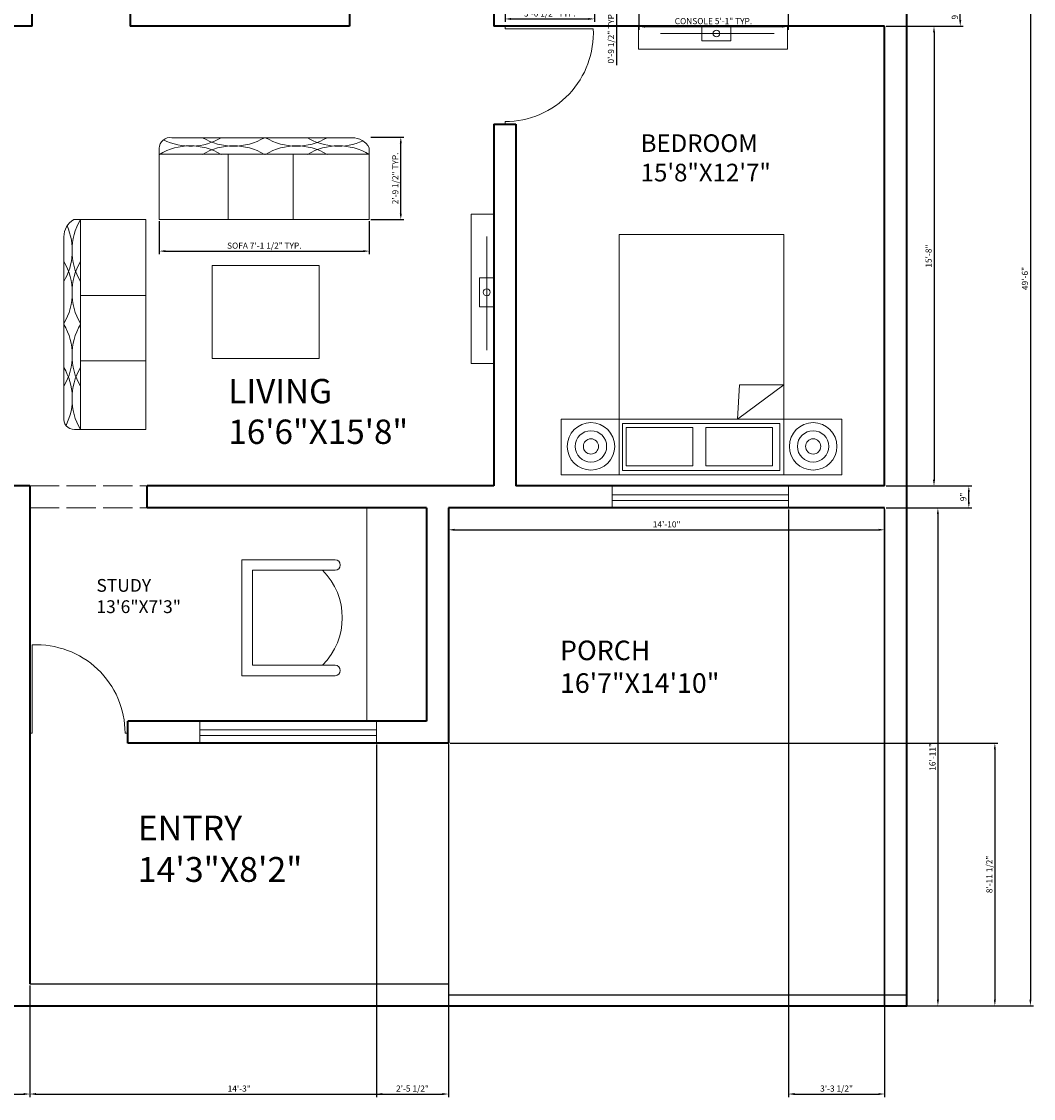
# Model space of a CAD drawing. Units: inches. Extents: x 808 to 1433, y 803 to 1556.
# Tile 2 of 4: x 1020 to 1433, y 803 to 1243. Entities that reach past the tile are written whole.
import ezdxf

# ---------------------------------------------------------------- set-up
doc = ezdxf.new("R2010")
doc.units = ezdxf.units.IN
doc.linetypes.add('ACAD_ISO02W100', pattern=[15, 12, -3])
for name, color, linetype, lineweight in [('A-ANNO-DIMS', 7, 'Continuous', 13), ('A-AREA-IDEN', 7, 'Continuous', 18), ('A-FLOR', 7, 'Continuous', 25), ('A-FLOR-CASE', 7, 'Continuous', 18), ('A-FLOR-OVHD', 7, 'ACAD_ISO02W100', 13), ('A-WALL', 7, 'Continuous', 35)]:
    doc.layers.add(name, color=color, linetype=linetype, lineweight=lineweight)
for name, color, linetype, lineweight, true_color in [('A-DOOR', 251, 'Continuous', 18, 0x636466), ('A-FURN', 251, 'Continuous', 13, 0x636466), ('A-GLAZ', 251, 'Continuous', 18, 0x636466)]:
    doc.layers.add(name, color=color, linetype=linetype, lineweight=lineweight, true_color=true_color)
doc.styles.get("Standard").update_dxf_attribs({"font": 'arial.ttf'})
doc.dimstyles.new('ISO-25', dxfattribs={"dimtxt": 2.5, "dimasz": 2.5, "dimexe": 1.25, "dimexo": 0.625, "dimtad": 1, "dimdec": 0, "dimlunit": 3, "dimtxsty": 'Standard', "dimcen": 2.5, "dimadec": 0, "dimazin": 0, "dimtfac": 1, "dimtdec": 0, "dimtmove": 0, "dimatfit": 3, "dimfxl": 1, "dimarcsym": 0})

# ---------------------------------------------------------------- blocks, each defined once
blk = doc.blocks.new('*D2')
at = {"layer": 'A-ANNO-DIMS', "color": 0, "lineweight": -2, "transparency": 16777216}
for p, q in [((1381.5, 1435.07), (1432.64, 1435.07)), ((1431.39, 1432.57), (1431.39, 843.57)), ((1381.5, 841.07), (1432.64, 841.07))]:
    blk.add_line(p, q, dxfattribs=at)
at = {"layer": 'A-ANNO-DIMS', "color": 0, "transparency": 16777216}
for points in [[(1430.97, 1432.57), (1431.8, 1432.57), (1431.39, 1435.07)], [(1430.97, 843.57), (1431.8, 843.57), (1431.39, 841.07)]]:
    blk.add_solid(points, dxfattribs=at)
at = {"layer": 'Defpoints', "color": 0, "transparency": 16777216}
for p in [(1380.88, 1435.07), (1380.88, 841.07), (1431.39, 841.07)]:
    blk.add_point(p, dxfattribs=at)
at = {"layer": 'A-ANNO-DIMS', "color": 0, "transparency": 16777216, "insert": (1429.48, 1138.07), "char_height": 2.5, "attachment_point": 5, "rotation": 90}
blk.add_mtext('49\'-6"', dxfattribs=at)
blk = doc.blocks.new('*D21')
at = {"layer": 'A-ANNO-DIMS', "color": 0, "lineweight": -2, "transparency": 16777216}
for p, q in [((1372.5, 1250.07), (1404, 1250.07)), ((1402.75, 1243.57), (1402.75, 1247.57)), ((1372.5, 1241.07), (1404, 1241.07))]:
    blk.add_line(p, q, dxfattribs=at)
at = {"layer": 'A-ANNO-DIMS', "color": 0, "transparency": 16777216}
for points in [[(1402.33, 1247.57), (1403.16, 1247.57), (1402.75, 1250.07)], [(1402.33, 1243.57), (1403.16, 1243.57), (1402.75, 1241.07)]]:
    blk.add_solid(points, dxfattribs=at)
at = {"layer": 'Defpoints', "color": 0, "transparency": 16777216}
for p in [(1371.88, 1250.07), (1402.75, 1250.07), (1371.88, 1241.07)]:
    blk.add_point(p, dxfattribs=at)
at = {"layer": 'A-ANNO-DIMS', "color": 0, "transparency": 16777216, "insert": (1400.85, 1245.57), "char_height": 2.5, "attachment_point": 5, "rotation": 90}
blk.add_mtext('9"', dxfattribs=at)
blk = doc.blocks.new('*D22')
at = {"layer": 'A-ANNO-DIMS', "color": 0, "lineweight": -2, "transparency": 16777216}
for p, q in [((1372.5, 1053.37), (1407.5, 1053.37)), ((1406.25, 1046.87), (1406.25, 1050.87)), ((1372.5, 1044.37), (1407.5, 1044.37))]:
    blk.add_line(p, q, dxfattribs=at)
at = {"layer": 'A-ANNO-DIMS', "color": 0, "transparency": 16777216}
for points in [[(1405.83, 1050.87), (1406.66, 1050.87), (1406.25, 1053.37)], [(1405.83, 1046.87), (1406.66, 1046.87), (1406.25, 1044.37)]]:
    blk.add_solid(points, dxfattribs=at)
at = {"layer": 'Defpoints', "color": 0, "transparency": 16777216}
for p in [(1371.88, 1053.37), (1406.25, 1053.37), (1371.88, 1044.37)]:
    blk.add_point(p, dxfattribs=at)
at = {"layer": 'A-ANNO-DIMS', "color": 0, "transparency": 16777216, "insert": (1404.34, 1048.87), "char_height": 2.5, "attachment_point": 5, "rotation": 90}
blk.add_mtext('9"', dxfattribs=at)
blk = doc.blocks.new('*D23')
at = {"layer": 'A-ANNO-DIMS', "color": 0, "lineweight": -2, "transparency": 16777216}
for p, q in [((1193.88, 1043.75), (1193.88, 1034.21)), ((1371.88, 1043.75), (1371.88, 1034.21)), ((1196.38, 1035.46), (1369.38, 1035.46))]:
    blk.add_line(p, q, dxfattribs=at)
at = {"layer": 'A-ANNO-DIMS', "color": 0, "transparency": 16777216}
for points in [[(1196.38, 1035.88), (1196.38, 1035.04), (1193.88, 1035.46)], [(1369.38, 1035.88), (1369.38, 1035.04), (1371.88, 1035.46)]]:
    blk.add_solid(points, dxfattribs=at)
at = {"layer": 'Defpoints', "color": 0, "transparency": 16777216}
for p in [(1193.88, 1044.37), (1371.88, 1044.37), (1371.88, 1035.46)]:
    blk.add_point(p, dxfattribs=at)
at = {"layer": 'A-ANNO-DIMS', "color": 0, "transparency": 16777216, "insert": (1282.88, 1037.36), "char_height": 2.5, "attachment_point": 5}
blk.add_mtext('14\'-10"', dxfattribs=at)
blk = doc.blocks.new('*D24')
at = {"layer": 'A-ANNO-DIMS', "color": 0, "lineweight": -2, "transparency": 16777216}
for p, q in [((1381.5, 1044.37), (1394.88, 1044.37)), ((1393.63, 1041.87), (1393.63, 843.57)), ((1381.5, 841.07), (1394.88, 841.07))]:
    blk.add_line(p, q, dxfattribs=at)
at = {"layer": 'A-ANNO-DIMS', "color": 0, "transparency": 16777216}
for points in [[(1393.21, 1041.87), (1394.04, 1041.87), (1393.63, 1044.37)], [(1393.21, 843.57), (1394.04, 843.57), (1393.63, 841.07)]]:
    blk.add_solid(points, dxfattribs=at)
at = {"layer": 'Defpoints', "color": 0, "transparency": 16777216}
for p in [(1380.88, 1044.37), (1380.88, 841.07), (1393.63, 841.07)]:
    blk.add_point(p, dxfattribs=at)
at = {"layer": 'A-ANNO-DIMS', "color": 0, "transparency": 16777216, "insert": (1391.73, 942.72), "char_height": 2.5, "attachment_point": 5, "rotation": 90}
blk.add_mtext('16\'-11"', dxfattribs=at)
blk = doc.blocks.new('*D25')
at = {"layer": 'A-ANNO-DIMS', "color": 0, "lineweight": -2, "transparency": 16777216}
for p, q in [((1381.5, 1241.07), (1393.29, 1241.07)), ((1392.04, 1238.57), (1392.04, 1055.87)), ((1381.5, 1053.37), (1393.29, 1053.37))]:
    blk.add_line(p, q, dxfattribs=at)
at = {"layer": 'A-ANNO-DIMS', "color": 0, "transparency": 16777216}
for points in [[(1391.62, 1238.57), (1392.45, 1238.57), (1392.04, 1241.07)], [(1391.62, 1055.87), (1392.45, 1055.87), (1392.04, 1053.37)]]:
    blk.add_solid(points, dxfattribs=at)
at = {"layer": 'Defpoints', "color": 0, "transparency": 16777216}
for p in [(1380.88, 1241.07), (1380.88, 1053.37), (1392.04, 1053.37)]:
    blk.add_point(p, dxfattribs=at)
at = {"layer": 'A-ANNO-DIMS', "color": 0, "transparency": 16777216, "insert": (1390.14, 1147.22), "char_height": 2.5, "attachment_point": 5, "rotation": 90}
blk.add_mtext('15\'-8"', dxfattribs=at)
blk = doc.blocks.new('BED-DOUBLE-NIGHTSTANDS')
for p, q in [((23.66, 75.46), (90.98, 75.46)), ((72.01, 75.46), (90.98, 61.39)), ((72.82, 61.39), (72.01, 75.46)), ((90.98, 61.39), (72.82, 61.39))]:
    blk.add_line(p, q)
for points in [[(23.66, 98.16), (0, 98.16), (0, 75.46), (23.66, 75.46)], [(23.66, 0), (90.98, 0), (90.98, 98.16), (23.66, 98.16)], [(114.63, 98.16), (90.98, 98.16), (90.98, 75.46), (114.63, 75.46)], [(25.04, 77.24), (89.23, 77.24), (89.23, 96.41), (25.04, 96.41)], [(26.57, 78.89), (53.84, 78.89), (53.84, 94.57), (26.57, 94.57)], [(59.07, 78.89), (86.35, 78.89), (86.35, 94.57), (59.07, 94.57)]]:
    blk.add_lwpolyline(points, close=True)
for centre, radius in [((12.19, 86.58), 9.7), ((12.19, 86.58), 6.41), ((102.89, 86.58), 9.7), ((102.89, 86.58), 6.41), ((12.19, 86.58), 3.11), ((102.89, 86.58), 3.11)]:
    blk.add_circle(centre, radius)
blk = doc.blocks.new('SOFA-3SEAT')
for p, q in [((78.71, 33.47), (5.06, 33.47)), ((0, 29.12), (0, 26.67)), ((28.12, 0), (28.12, 26.67)), ((54.7, 0), (54.7, 26.67)), ((85.72, 26.67), (85.72, 29.39))]:
    blk.add_line(p, q)
blk.add_lwpolyline([(0, 0), (85.72, 0), (85.72, 26.67), (0, 26.67)], close=True)
for centre, radius, start, end in [((4.4, 29.12), 4.4, 81.2898, 180), ((12.64, 54.74), 24.74, 243.6614, 300.7197), ((30.31, 54.74), 24.74, 239.2803, 300.7197), ((55.93, 54.74), 24.74, 239.2803, 300.7197), ((73.08, 54.74), 24.74, 239.2803, 294.0125), ((78.71, 25.4), 8.06, 29.6577, 90), ((12.64, 5.39), 24.74, 59.2803, 120.7197), ((30.31, 5.39), 24.74, 59.2803, 120.7197), ((55.93, 5.39), 24.74, 59.2803, 120.7197), ((73.08, 5.39), 24.74, 59.2803, 120.7197)]:
    blk.add_arc(centre, radius, start, end)
blk = doc.blocks.new('MEDIA-CONSOLE')
for q in [(6.39, 51.9), (6.39, 5.5)]:
    blk.add_line((6.39, 23.14), q)
for points in [[(9.33, 60.92), (0, 60.92), (0, 0), (9.33, 0)], [(9.33, 35.01), (3.45, 35.01), (3.45, 23.14), (9.33, 23.14)]]:
    blk.add_lwpolyline(points, close=True)
blk.add_circle((6.39, 29.07), 1.39)
blk = doc.blocks.new('WIN-72')
for points in [[(0, 0), (72, 0), (72, 9), (0, 9)], [(0, 5.39), (72, 5.39), (72, 3.12), (0, 3.12)]]:
    blk.add_lwpolyline(points, close=True)
blk = doc.blocks.new('DOOR-40')
for p, q in [((0, 40), (0, 38.9)), ((0, 1), (36, 1)), ((0, 1), (0, 0))]:
    blk.add_line(p, q)
blk.add_arc((0, 2.85), 36.05, 357.0527, 90)
blk = doc.blocks.new('*D48')
at = {"layer": 'A-ANNO-DIMS', "color": 0, "lineweight": -2, "transparency": 16777216}
for p, q in [((1216.91, 1249.44), (1216.91, 1242.82)), ((1253.42, 1249.44), (1253.42, 1242.82)), ((1219.41, 1244.07), (1250.92, 1244.07))]:
    blk.add_line(p, q, dxfattribs=at)
at = {"layer": 'A-ANNO-DIMS', "color": 0, "transparency": 16777216}
for points in [[(1219.41, 1244.48), (1219.41, 1243.65), (1216.91, 1244.07)], [(1250.92, 1244.48), (1250.92, 1243.65), (1253.42, 1244.07)]]:
    blk.add_solid(points, dxfattribs=at)
at = {"layer": 'Defpoints', "color": 0, "transparency": 16777216}
for p in [(1216.91, 1250.07), (1253.42, 1250.07), (1253.42, 1244.07)]:
    blk.add_point(p, dxfattribs=at)
at = {"layer": 'A-ANNO-DIMS', "color": 0, "transparency": 16777216, "insert": (1235.17, 1245.98), "char_height": 2.5, "attachment_point": 5}
blk.add_mtext('3\'-0 1/2" TYP.', dxfattribs=at)
blk = doc.blocks.new('*D55')
at = {"layer": 'A-ANNO-DIMS', "color": 0, "lineweight": -2, "transparency": 16777216}
for p, q in [((1075.78, 1161.49), (1075.78, 1148.01)), ((1161.5, 1161.49), (1161.5, 1148.01)), ((1078.28, 1149.26), (1159, 1149.26))]:
    blk.add_line(p, q, dxfattribs=at)
at = {"layer": 'A-ANNO-DIMS', "color": 0, "transparency": 16777216}
for points in [[(1078.28, 1149.67), (1078.28, 1148.84), (1075.78, 1149.26)], [(1159, 1149.67), (1159, 1148.84), (1161.5, 1149.26)]]:
    blk.add_solid(points, dxfattribs=at)
at = {"layer": 'Defpoints', "color": 0, "transparency": 16777216}
for p in [(1075.78, 1162.11), (1161.5, 1162.11), (1161.5, 1149.26)]:
    blk.add_point(p, dxfattribs=at)
at = {"layer": 'A-ANNO-DIMS', "color": 0, "transparency": 16777216, "insert": (1118.64, 1151.17), "char_height": 2.5, "attachment_point": 5}
blk.add_mtext('SOFA 7\'-1 1/2" TYP.', dxfattribs=at)
blk = doc.blocks.new('*D56')
at = {"layer": 'A-ANNO-DIMS', "color": 0, "lineweight": -2, "transparency": 16777216}
for p, q in [((1162.13, 1195.78), (1175.61, 1195.78)), ((1174.36, 1164.61), (1174.36, 1193.28)), ((1162.13, 1162.11), (1175.61, 1162.11))]:
    blk.add_line(p, q, dxfattribs=at)
at = {"layer": 'A-ANNO-DIMS', "color": 0, "transparency": 16777216}
for points in [[(1173.94, 1193.28), (1174.78, 1193.28), (1174.36, 1195.78)], [(1173.94, 1164.61), (1174.78, 1164.61), (1174.36, 1162.11)]]:
    blk.add_solid(points, dxfattribs=at)
at = {"layer": 'Defpoints', "color": 0, "transparency": 16777216}
for p in [(1161.5, 1195.78), (1174.36, 1195.78), (1161.5, 1162.11)]:
    blk.add_point(p, dxfattribs=at)
at = {"layer": 'A-ANNO-DIMS', "color": 0, "transparency": 16777216, "insert": (1172.44, 1178.95), "char_height": 2.5, "attachment_point": 5, "rotation": 90}
blk.add_mtext('2\'-9 1/2" TYP.', dxfattribs=at)
blk = doc.blocks.new('*D57')
at = {"layer": 'A-ANNO-DIMS', "color": 0, "lineweight": -2, "transparency": 16777216}
for p, q in [((1271.53, 1249.44), (1271.53, 1239.68)), ((1332.45, 1249.44), (1332.45, 1239.68)), ((1274.03, 1240.93), (1329.95, 1240.93))]:
    blk.add_line(p, q, dxfattribs=at)
at = {"layer": 'A-ANNO-DIMS', "color": 0, "transparency": 16777216}
for points in [[(1274.03, 1241.35), (1274.03, 1240.51), (1271.53, 1240.93)], [(1329.95, 1241.35), (1329.95, 1240.51), (1332.45, 1240.93)]]:
    blk.add_solid(points, dxfattribs=at)
at = {"layer": 'Defpoints', "color": 0, "transparency": 16777216}
for p in [(1271.53, 1250.07), (1332.45, 1250.07), (1332.45, 1240.93)]:
    blk.add_point(p, dxfattribs=at)
at = {"layer": 'A-ANNO-DIMS', "color": 0, "transparency": 16777216, "insert": (1301.99, 1242.85), "char_height": 2.5, "attachment_point": 5}
blk.add_mtext('CONSOLE 5\'-1" TYP.', dxfattribs=at)
blk = doc.blocks.new('*D58')
at = {"layer": 'A-ANNO-DIMS', "color": 0, "lineweight": -2, "transparency": 16777216}
for p, q in [((1270.91, 1259.4), (1261.14, 1259.4)), ((1262.39, 1256.9), (1262.39, 1252.57)), ((1270.91, 1250.07), (1261.14, 1250.07)), ((1262.39, 1250.07), (1262.39, 1225.25))]:
    blk.add_line(p, q, dxfattribs=at)
at = {"layer": 'A-ANNO-DIMS', "color": 0, "transparency": 16777216}
for points in [[(1261.98, 1256.9), (1262.81, 1256.9), (1262.39, 1259.4)], [(1261.98, 1252.57), (1262.81, 1252.57), (1262.39, 1250.07)]]:
    blk.add_solid(points, dxfattribs=at)
at = {"layer": 'Defpoints', "color": 0, "transparency": 16777216}
for p in [(1271.53, 1259.4), (1262.39, 1250.07), (1271.53, 1250.07)]:
    blk.add_point(p, dxfattribs=at)
at = {"layer": 'A-ANNO-DIMS', "color": 0, "transparency": 16777216, "insert": (1260.48, 1236.41), "char_height": 2.5, "attachment_point": 5, "rotation": 90}
blk.add_mtext('0\'-9 1/2" TYP.', dxfattribs=at)
blk = doc.blocks.new('*D66')
at = {"layer": 'A-ANNO-DIMS', "color": 0, "lineweight": -2, "transparency": 16777216}
for p, q in [((1022.88, 849.44), (1022.88, 803.82)), ((971.87, 840.44), (971.87, 803.82)), ((974.37, 805.07), (1020.38, 805.07))]:
    blk.add_line(p, q, dxfattribs=at)
at = {"layer": 'A-ANNO-DIMS', "color": 0, "transparency": 16777216}
for points in [[(974.37, 805.48), (974.37, 804.65), (971.87, 805.07)], [(1020.38, 805.48), (1020.38, 804.65), (1022.88, 805.07)]]:
    blk.add_solid(points, dxfattribs=at)
at = {"layer": 'Defpoints', "color": 0, "transparency": 16777216}
for p in [(1022.88, 850.07), (971.87, 841.07), (1022.88, 805.07)]:
    blk.add_point(p, dxfattribs=at)
at = {"layer": 'A-ANNO-DIMS', "color": 0, "transparency": 16777216, "insert": (997.38, 806.97), "char_height": 2.5, "attachment_point": 5}
blk.add_mtext('4\'-3"', dxfattribs=at)
blk = doc.blocks.new('*D67')
at = {"layer": 'A-ANNO-DIMS', "color": 0, "lineweight": -2, "transparency": 16777216}
for p, q in [((1022.88, 849.44), (1022.88, 803.82)), ((1193.88, 840.44), (1193.88, 803.82)), ((1025.38, 805.07), (1191.38, 805.07))]:
    blk.add_line(p, q, dxfattribs=at)
at = {"layer": 'A-ANNO-DIMS', "color": 0, "transparency": 16777216}
for points in [[(1025.38, 805.48), (1025.38, 804.65), (1022.88, 805.07)], [(1191.38, 805.48), (1191.38, 804.65), (1193.88, 805.07)]]:
    blk.add_solid(points, dxfattribs=at)
at = {"layer": 'Defpoints', "color": 0, "transparency": 16777216}
for p in [(1022.88, 850.07), (1193.88, 841.07), (1193.88, 805.07)]:
    blk.add_point(p, dxfattribs=at)
at = {"layer": 'A-ANNO-DIMS', "color": 0, "transparency": 16777216, "insert": (1108.38, 806.97), "char_height": 2.5, "attachment_point": 5}
blk.add_mtext('14\'-3"', dxfattribs=at)
blk = doc.blocks.new('*D70')
at = {"layer": 'A-ANNO-DIMS', "color": 0, "lineweight": -2, "transparency": 16777216}
for p, q in [((1164.38, 947.75), (1164.38, 803.82)), ((1193.88, 947.75), (1193.88, 803.82)), ((1166.88, 805.07), (1191.38, 805.07))]:
    blk.add_line(p, q, dxfattribs=at)
at = {"layer": 'A-ANNO-DIMS', "color": 0, "transparency": 16777216}
for points in [[(1166.88, 805.48), (1166.88, 804.65), (1164.38, 805.07)], [(1191.38, 805.48), (1191.38, 804.65), (1193.88, 805.07)]]:
    blk.add_solid(points, dxfattribs=at)
at = {"layer": 'Defpoints', "color": 0, "transparency": 16777216}
for p in [(1164.38, 948.37), (1193.88, 948.37), (1193.88, 805.07)]:
    blk.add_point(p, dxfattribs=at)
at = {"layer": 'A-ANNO-DIMS', "color": 0, "transparency": 16777216, "insert": (1179.13, 806.98), "char_height": 2.5, "attachment_point": 5}
blk.add_mtext('2\'-5 1/2"', dxfattribs=at)
blk = doc.blocks.new('*D71')
at = {"layer": 'A-ANNO-DIMS', "color": 0, "lineweight": -2, "transparency": 16777216}
for p, q in [((1194.5, 948.37), (1418.13, 948.37)), ((1416.88, 945.87), (1416.88, 843.57)), ((1194.5, 841.07), (1418.13, 841.07))]:
    blk.add_line(p, q, dxfattribs=at)
at = {"layer": 'A-ANNO-DIMS', "color": 0, "transparency": 16777216}
for points in [[(1416.46, 945.87), (1417.3, 945.87), (1416.88, 948.37)], [(1416.46, 843.57), (1417.3, 843.57), (1416.88, 841.07)]]:
    blk.add_solid(points, dxfattribs=at)
at = {"layer": 'Defpoints', "color": 0, "transparency": 16777216}
for p in [(1193.88, 948.37), (1193.88, 841.07), (1416.88, 841.07)]:
    blk.add_point(p, dxfattribs=at)
at = {"layer": 'A-ANNO-DIMS', "color": 0, "transparency": 16777216, "insert": (1414.96, 894.72), "char_height": 2.5, "attachment_point": 5, "rotation": 90}
blk.add_mtext('8\'-11 1/2"', dxfattribs=at)
blk = doc.blocks.new('*D74')
at = {"layer": 'A-ANNO-DIMS', "color": 0, "lineweight": -2, "transparency": 16777216}
for p, q in [((1332.63, 1043.75), (1332.63, 803.82)), ((1371.88, 1043.75), (1371.88, 803.82)), ((1335.13, 805.07), (1369.38, 805.07))]:
    blk.add_line(p, q, dxfattribs=at)
at = {"layer": 'A-ANNO-DIMS', "color": 0, "transparency": 16777216}
for points in [[(1335.13, 805.48), (1335.13, 804.65), (1332.63, 805.07)], [(1369.38, 805.48), (1369.38, 804.65), (1371.88, 805.07)]]:
    blk.add_solid(points, dxfattribs=at)
at = {"layer": 'Defpoints', "color": 0, "transparency": 16777216}
for p in [(1332.63, 1044.37), (1371.88, 1044.37), (1371.88, 805.07)]:
    blk.add_point(p, dxfattribs=at)
at = {"layer": 'A-ANNO-DIMS', "color": 0, "transparency": 16777216, "insert": (1352.25, 806.98), "char_height": 2.5, "attachment_point": 5}
blk.add_mtext('3\'-3 1/2"', dxfattribs=at)

msp = doc.modelspace()

# ---------------------------------------------------------------- linework, layer by layer
at = {"layer": 'A-FLOR'}
for p, q in [((1371.88, 841.07), (1371.88, 1044.37)), ((1022.88, 850.07), (1193.88, 850.07)), ((1193.88, 850.07), (1193.88, 841.07)), ((1193.88, 845.57), (1380.88, 845.57))]:
    msp.add_line(p, q, dxfattribs=at)
at = {"layer": 'A-FLOR-CASE'}
msp.add_line((1160.52, 1044.37), (1160.52, 957.37), dxfattribs=at)
at = {"layer": 'A-FLOR-OVHD'}
for p, q in [((1022.88, 1053.37), (1070.88, 1053.37)), ((1022.88, 1044.37), (1070.88, 1044.37)), ((1193.88, 948.37), (1193.88, 850.07))]:
    msp.add_line(p, q, dxfattribs=at)
at = {"layer": 'A-FURN'}
msp.add_lwpolyline([(1097.3, 1105.45), (1140.99, 1105.45), (1140.99, 1143.45), (1097.3, 1143.45)], close=True, dxfattribs=at)
for points in [[(1147.52, 1023.22), (1109.48, 1023.22), (1109.48, 975.88), (1147.52, 975.88)], [(1147.52, 1018.92), (1113.78, 1018.92), (1113.78, 980.19), (1147.52, 980.19)]]:
    msp.add_lwpolyline(points, dxfattribs=at)
for centre, radius, start, end in [((1147.52, 1021.07), 2.15, 270, 90), ((1123.08, 999.55), 27.39, 315, 45), ((1147.52, 978.03), 2.15, 270, 90)]:
    msp.add_arc(centre, radius, start, end, dxfattribs=at)
at = {"layer": 'A-WALL'}
for p, q in [((1380.88, 841.07), (1380.88, 1435.07)), ((1153.38, 1332.07), (1153.38, 1241.07)), ((1023.88, 1241.07), (1023.88, 1250.07)), ((1063.88, 1250.07), (1063.88, 1241.07)), ((1212.38, 1250.07), (1212.38, 1241.07)), ((1023.88, 1241.07), (863.88, 1241.07)), ((1153.38, 1241.07), (1063.88, 1241.07)), ((1371.88, 1241.07), (1212.38, 1241.07)), ((1371.88, 1053.37), (1371.88, 1241.07)), ((1212.38, 1201.07), (1221.38, 1201.07)), ((1212.38, 1201.07), (1212.38, 1053.37)), ((1221.38, 1201.07), (1221.38, 1053.37)), ((1022.88, 1053.37), (1013.88, 1053.37)), ((1022.88, 1053.37), (1022.88, 948.37)), ((1212.38, 1053.37), (1070.88, 1053.37)), ((1070.88, 1044.37), (1070.88, 1053.37)), ((1371.88, 1053.37), (1221.38, 1053.37)), ((1184.88, 1044.37), (1070.88, 1044.37)), ((1184.88, 1044.37), (1184.88, 957.37)), ((1371.88, 1044.37), (1193.88, 1044.37)), ((1193.88, 1044.37), (1193.88, 948.37)), ((1184.88, 957.37), (1062.88, 957.37)), ((1062.88, 948.37), (1062.88, 957.37)), ((1022.88, 948.37), (1022.88, 850.07)), ((1193.88, 948.37), (1062.88, 948.37)), ((854.88, 841.07), (1380.88, 841.07))]:
    msp.add_line(p, q, dxfattribs=at)

# ---------------------------------------------------------------- block references
at = {"layer": 'A-DOOR', "extrusion": (0, 0, -1), "zscale": -1}
for p, rotation in [((-1216.91, 1241.07), 180), ((-1022.88, 952.43), 90.00000000000244)]:
    msp.add_blockref('DOOR-40', p, dxfattribs=dict(at, rotation=rotation))
at = {"layer": 'A-FURN'}
for name, p, rotation in [('MEDIA-CONSOLE', (1332.28, 1231.73), 89.9999999999995), ('SOFA-3SEAT', (1070.26, 1076.4), 89.9999999999992)]:
    msp.add_blockref(name, p, dxfattribs=dict(at, rotation=rotation))
for name, p in [('SOFA-3SEAT', (1075.78, 1162.11)), ('MEDIA-CONSOLE', (1203.05, 1103.38))]:
    msp.add_blockref(name, p, dxfattribs=at)
at = {"layer": 'A-FURN', "extrusion": (0, 0, -1), "zscale": -1, "rotation": 180}
msp.add_blockref('BED-DOUBLE-NIGHTSTANDS', (-1239.8, 1156.1), dxfattribs=at)
at = {"layer": 'A-GLAZ'}
for p in [(1260.63, 1044.37), (1092.38, 948.37)]:
    msp.add_blockref('WIN-72', p, dxfattribs=at)

# ---------------------------------------------------------------- texts
at = {"layer": 'A-AREA-IDEN', "attachment_point": 1}
for s, width, gutter_width, insert, char_height in [('BEDROOM\\P15\'8"X12\'7"', 312.5212, 36.01, (1272.28, 1196.94), 7.2014), ('LIVING\\P16\'6"X15\'8"', 257.4052, 49.75, (1103.97, 1097.06), 9.9501), ('STUDY\\P13\'6"X7\'3"', 73.6255, 26.08, (1050.1, 1015.37), 5.216), ('PORCH\\P16\'7"X14\'10"', 200.0204, 40, (1239.36, 990.22), 8), ('ENTRY\\P14\'3"X8\'2"', 213.4458, 50.75, (1066.97, 918.76), 10.15)]:
    msp.add_mtext_dynamic_manual_height_columns(s, width=width, gutter_width=gutter_width, heights=[0], dxfattribs=dict(at, insert=insert, char_height=char_height))

# ---------------------------------------------------------------- dimensions: what is measured, and where the dimension line sits
at = {"layer": 'A-ANNO-DIMS'}
for base, p1, p2, override, picture, middle in [((1431.39, 841.07), (1380.88, 1435.07), (1380.88, 841.07), {"dimclrd": 0, "dimclre": 0, "dimclrt": 0}, '*D2', (1429.48, 1138.07)), ((1402.75, 1250.07), (1371.88, 1241.07), (1371.88, 1250.07), {"dimclrd": 0, "dimclre": 0, "dimclrt": 0}, '*D21', (1400.85, 1245.57)), ((1392.04, 1053.37), (1380.88, 1241.07), (1380.88, 1053.37), {"dimclrd": 0, "dimclre": 0, "dimclrt": 0}, '*D25', (1390.14, 1147.22)), ((1406.25, 1053.37), (1371.88, 1044.37), (1371.88, 1053.37), {"dimclrd": 0, "dimclre": 0, "dimclrt": 0}, '*D22', (1404.34, 1048.87)), ((1393.63, 841.07), (1380.88, 1044.37), (1380.88, 841.07), {"dimclrd": 0, "dimclre": 0, "dimclrt": 0}, '*D24', (1391.73, 942.72)), ((1416.88, 841.07), (1193.88, 948.37), (1193.88, 841.07), {"dimdec": 1, "dimlfac": 1, "dimrnd": 0, "dimzin": 1, "dimdsep": 46, "dimlunit": 4, "dimfrac": 2}, '*D71', (1414.96, 894.72))]:
    dim = msp.add_linear_dim(base=base, p1=p1, p2=p2, angle=90, dimstyle='ISO-25', override=override, dxfattribs=at)
    dim.commit()
    dim.dimension.update_dxf_attribs({"geometry": picture, "text_midpoint": middle})
for base, p1, p2, angle, text, picture, middle in [((1262.39, 1250.07), (1271.53, 1259.4), (1271.53, 1250.07), 270, '<> TYP.', '*D58', (1260.48, 1236.41)), ((1332.45, 1240.93), (1271.53, 1250.07), (1332.45, 1250.07), 0, 'CONSOLE <> TYP.', '*D57', (1301.99, 1242.85)), ((1174.36, 1195.78), (1161.5, 1162.11), (1161.5, 1195.78), 90, '<> TYP.', '*D56', (1172.44, 1178.95))]:
    dim = msp.add_linear_dim(base=base, p1=p1, p2=p2, angle=angle, text=text, dimstyle='ISO-25', override={"dimdec": 1, "dimlfac": 1, "dimrnd": 0, "dimzin": 1, "dimdsep": 46, "dimlunit": 4, "dimfrac": 2}, dxfattribs=at)
    dim.commit()
    dim.dimension.update_dxf_attribs({"geometry": picture, "text_midpoint": middle})
for base, p1, p2, text, picture, middle in [((1253.42, 1244.07), (1216.91, 1250.07), (1253.42, 1250.07), '<> TYP.', '*D48', (1235.17, 1245.98)), ((1161.5, 1149.26), (1075.78, 1162.11), (1161.5, 1162.11), 'SOFA <> TYP.', '*D55', (1118.64, 1151.17))]:
    dim = msp.add_linear_dim(base=base, p1=p1, p2=p2, text=text, dimstyle='ISO-25', override={"dimdec": 1, "dimlfac": 1, "dimrnd": 0, "dimzin": 1, "dimdsep": 46, "dimlunit": 4, "dimfrac": 2}, dxfattribs=at)
    dim.commit()
    dim.dimension.update_dxf_attribs({"geometry": picture, "text_midpoint": middle})
for base, p1, p2, override, picture, middle in [((1371.88, 1035.46), (1193.88, 1044.37), (1371.88, 1044.37), {"dimclrd": 0, "dimclre": 0, "dimclrt": 0}, '*D23', (1282.88, 1037.36)), ((1371.879538, 805.06624), (1332.629538, 1044.371443), (1371.879538, 1044.371443), {"dimdec": 1, "dimlfac": 1, "dimrnd": 0, "dimzin": 1, "dimdsep": 46, "dimlunit": 4, "dimfrac": 2}, '*D74', (1352.254538, 806.98472568)), ((1193.88, 805.07), (1164.38, 948.37), (1193.88, 948.37), {"dimdec": 1, "dimlfac": 1, "dimrnd": 0, "dimzin": 1, "dimdsep": 46, "dimlunit": 4, "dimfrac": 2}, '*D70', (1179.13, 806.98)), ((1022.88, 805.07), (971.87, 841.07), (1022.88, 850.07), {"dimdec": 1, "dimlfac": 1, "dimrnd": 0, "dimzin": 1, "dimdsep": 46, "dimlunit": 4, "dimfrac": 2}, '*D66', (997.38, 806.97)), ((1193.88, 805.07), (1022.88, 850.07), (1193.88, 841.07), {"dimdec": 1, "dimlfac": 1, "dimrnd": 0, "dimzin": 1, "dimdsep": 46, "dimlunit": 4, "dimfrac": 2}, '*D67', (1108.38, 806.97))]:
    dim = msp.add_linear_dim(base=base, p1=p1, p2=p2, dimstyle='ISO-25', override=override, dxfattribs=at)
    dim.commit()
    dim.dimension.update_dxf_attribs({"geometry": picture, "text_midpoint": middle})

doc.saveas('drawing.dxf')
